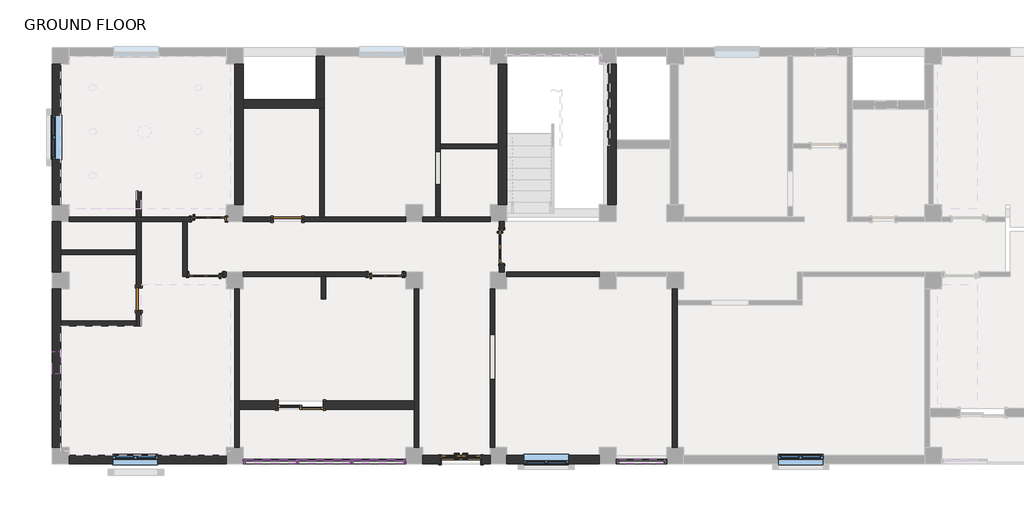
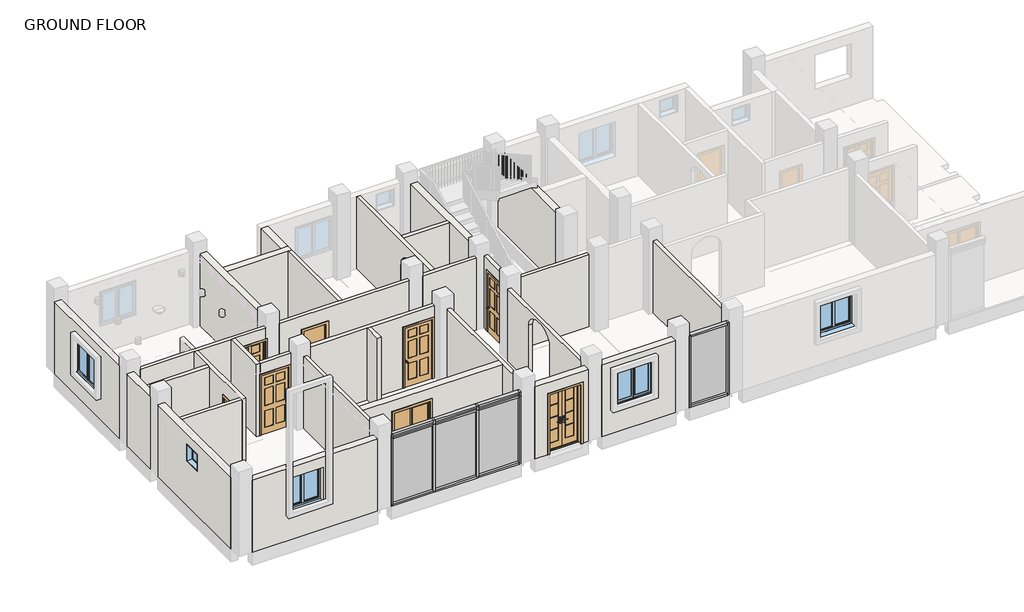
# One storey, part 1 of 5: 31 walls, 21 members, 8 doors, 7 plates, 5 windows.
"""IFC4 building model written with IfcOpenShell, lengths in millimetres."""

from ifc_helpers import new_model, si_unit, point, frame, origin, place, context, project, spatial, polyline, ellipse_curve, trimmed, outline, extrude, faceted_brep, transform, mapped, element, save
from ifc_brep_helpers import plane_surface, extruded_surface, advanced_brep
from components import door_double_sliding_4436dcad, door_exterior_double_full_glass_wood_clad_a9b2ee3b, door_c610b25b, door_03e3dfb5, single_flush_2_x_7_bath_room_door_025d1c86, door_e00f436c, member_f0fea5a5, member_ee409385, member_2b4cd6f1, member_0dc43c0c, member_71eb4692, member_9f3fc137, member_faf5b19b, member_68d3d74d, member_f51719be, member_c9ff5349, system_panel_glazed_7ffa2d15, system_panel_glazed_7e177a0b, system_panel_glazed_c89335d8, system_panel_glazed_a1658219, system_panel_glazed_dde0d99a, window_80340324, w2_0001_4_x_4_window_9dec5fc7

model = new_model("IFC4")

# Units and contexts
model_context = context("Model", 3, world=origin())
ifc_project = project(units=[si_unit("LENGTHUNIT", "METRE", prefix="MILLI")], contexts=[model_context])

# Site, building, storey
site = spatial("IfcSite", under=ifc_project)
building = spatial("IfcBuilding", under=site)
storey = spatial("IfcBuildingStorey", under=building, Name="GROUND FLOOR", Elevation=304.8)

# Doors
placement = place(None, origin())
door_double_sliding_shape = door_double_sliding_4436dcad(model_context)
element("IfcDoor", 1, ObjectType="Door-Double-Sliding", at=placement, inside=storey, context=model_context, shape_type="MappedRepresentation", body=[
    mapped(door_double_sliding_shape, transform((-8630.2456086, -9389.2679047, 304.8), x_axis=(-1.0, 0.0, 0.0), y_axis=(0.0, -1.0, 0.0), z_axis=(0.0, 0.0, 1.0))),
])
door_exterior_double_full_glass_wood_clad_shape = door_exterior_double_full_glass_wood_clad_a9b2ee3b(model_context)
element("IfcDoor", 2, ObjectType="Door-Exterior-Double-Full Glass-Wood_Clad", at=placement, inside=storey, context=model_context, shape_type="MappedRepresentation", body=[
    mapped(door_exterior_double_full_glass_wood_clad_shape, transform((-4274.1456086, -10998.9929047, 304.8), x_axis=(1.0, 0.0, 0.0), y_axis=(0.0, 1.0, 0.0), z_axis=(0.0, 0.0, 1.0))),
])
door_shape = door_c610b25b(model_context)
element("IfcDoor", 3, ObjectType="Door-Interior-Single-6_Panel-Wood : 36\" x 84\"", at=placement, inside=storey, context=model_context, shape_type="MappedRepresentation", body=[
    mapped(door_shape, transform((-6331.5456086, -5967.8544704, 304.8), x_axis=(1.0, 0.0, 0.0), y_axis=(0.0, 1.0, 0.0), z_axis=(0.0, 0.0, 1.0))),
])
element("IfcDoor", 4, ObjectType="Door-Interior-Single-6_Panel-Wood : 36\" x 84\"", at=placement, inside=storey, context=model_context, shape_type="MappedRepresentation", body=[
    mapped(door_shape, transform((-3172.4206086, -5215.3794704, 304.8), x_axis=(0.0, -1.0, 0.0), y_axis=(1.0, 0.0, 0.0), z_axis=(0.0, 0.0, 1.0))),
])
door_2_shape = door_03e3dfb5(model_context)
element("IfcDoor", 5, ObjectType="Door-Interior-Single-6_Panel-Wood : 36\" x 84\"", at=placement, inside=storey, context=model_context, shape_type="MappedRepresentation", body=[
    mapped(door_2_shape, transform((-11207.742897, -5967.8544704, 304.8), x_axis=(-1.0, 0.0, 0.0), y_axis=(0.0, -1.0, 0.0), z_axis=(0.0, 0.0, 1.0))),
])
element("IfcDoor", 6, ObjectType="Door-Interior-Single-6_Panel-Wood : 36\" x 84\"", at=placement, inside=storey, context=model_context, shape_type="MappedRepresentation", body=[
    mapped(door_2_shape, transform((-11132.1456086, -4462.9044704, 304.8), x_axis=(1.0, 0.0, 0.0), y_axis=(0.0, 1.0, 0.0), z_axis=(0.0, 0.0, 1.0))),
])
single_flush_2_x_7_bath_room_door_shape = single_flush_2_x_7_bath_room_door_025d1c86(model_context)
element("IfcDoor", 7, ObjectType="Single-Flush : 2' X 7' BATH ROOM DOOR", at=placement, inside=storey, context=model_context, shape_type="MappedRepresentation", body=[
    mapped(single_flush_2_x_7_bath_room_door_shape, transform((-13023.2401855, -6639.2659448, 304.8), x_axis=(0.0, 1.0, 0.0), y_axis=(-1.0, 0.0, 0.0), z_axis=(0.0, 0.0, 1.0))),
])
door_3_shape = door_e00f436c(model_context)
element("IfcDoor", 8, ObjectType="Single-Flush : bathroom 2'6\" door", at=placement, inside=storey, context=model_context, shape_type="MappedRepresentation", body=[
    mapped(door_3_shape, transform((-8985.8456086, -4466.0794704, 304.8), x_axis=(-1.0, 0.0, 0.0), y_axis=(0.0, -1.0, 0.0), z_axis=(0.0, 0.0, 1.0))),
])

# Members
member_shape = member_f0fea5a5(model_context)
element("IfcMember", 9, ObjectType="Rectangular Mullion : 2.5\" x 5\" rectangular", at=placement, inside=storey, context=model_context, shape_type="MappedRepresentation", body=[
    mapped(member_shape, transform((-8719.1456085, -11052.9679047, 304.8), x_axis=(1.0, 0.0, 0.0), y_axis=(0.0, -1.0, 0.0), z_axis=(0.0, 0.0, -1.0))),
])
element("IfcMember", 10, ObjectType="Rectangular Mullion : 2.5\" x 5\" rectangular", at=placement, inside=storey, context=model_context, shape_type="MappedRepresentation", body=[
    mapped(member_shape, transform((-7245.9456087, -11052.9679047, 304.8), x_axis=(1.0, 0.0, 0.0), y_axis=(0.0, -1.0, 0.0), z_axis=(0.0, 0.0, -1.0))),
])
member_2_shape = member_ee409385(model_context)
element("IfcMember", 11, ObjectType="Rectangular Mullion : 2.5\" x 5\" rectangular", at=placement, inside=storey, context=model_context, shape_type="MappedRepresentation", body=[
    mapped(member_2_shape, transform((-5772.7456086, -11052.9679047, 304.8), x_axis=(1.0, 0.0, 0.0), y_axis=(0.0, -1.0, 0.0), z_axis=(0.0, 0.0, -1.0))),
])
element("IfcMember", 12, ObjectType="Rectangular Mullion : 2.5\" x 5\" rectangular", at=placement, inside=storey, context=model_context, shape_type="MappedRepresentation", body=[
    mapped(member_2_shape, transform((-10192.3456086, -11052.9679047, 2743.2), x_axis=(-1.0, 0.0, 0.0), y_axis=(0.0, -1.0, 0.0), z_axis=(0.0, 0.0, 1.0))),
])
member_3_shape = member_2b4cd6f1(model_context)
element("IfcMember", 13, ObjectType="Rectangular Mullion : 2.5\" x 5\" rectangular", at=placement, inside=storey, context=model_context, shape_type="MappedRepresentation", body=[
    mapped(member_3_shape, transform((-5836.2456086, -11052.9679047, 2892.0191055), x_axis=(0.0, 0.0, 1.0), y_axis=(0.0, -1.0, 0.0), z_axis=(1.0, 0.0, 0.0))),
])
element("IfcMember", 14, ObjectType="Rectangular Mullion : 2.5\" x 5\" rectangular", at=placement, inside=storey, context=model_context, shape_type="MappedRepresentation", body=[
    mapped(member_3_shape, transform((-8750.8956085, -11052.9679047, 2892.0191055), x_axis=(0.0, 0.0, 1.0), y_axis=(0.0, -1.0, 0.0), z_axis=(1.0, 0.0, 0.0))),
])
element("IfcMember", 15, ObjectType="Rectangular Mullion : 2.5\" x 5\" rectangular", at=placement, inside=storey, context=model_context, shape_type="MappedRepresentation", body=[
    mapped(member_3_shape, transform((-10128.8456086, -11052.9679047, 304.8), x_axis=(0.0, 0.0, -1.0), y_axis=(0.0, -1.0, 0.0), z_axis=(-1.0, 0.0, 0.0))),
])
element("IfcMember", 16, ObjectType="Rectangular Mullion : 2.5\" x 5\" rectangular", at=placement, inside=storey, context=model_context, shape_type="MappedRepresentation", body=[
    mapped(member_3_shape, transform((-7214.1956087, -11052.9679047, 304.8), x_axis=(0.0, 0.0, -1.0), y_axis=(0.0, -1.0, 0.0), z_axis=(-1.0, 0.0, 0.0))),
])
member_4_shape = member_0dc43c0c(model_context)
element("IfcMember", 17, ObjectType="Rectangular Mullion : 2.5\" x 5\" rectangular", at=placement, inside=storey, context=model_context, shape_type="MappedRepresentation", body=[
    mapped(member_4_shape, transform((-7277.6956087, -11052.9679047, 2892.0191055), x_axis=(0.0, 0.0, 1.0), y_axis=(0.0, -1.0, 0.0), z_axis=(1.0, 0.0, 0.0))),
])
element("IfcMember", 18, ObjectType="Rectangular Mullion : 2.5\" x 5\" rectangular", at=placement, inside=storey, context=model_context, shape_type="MappedRepresentation", body=[
    mapped(member_4_shape, transform((-8687.3956085, -11052.9679047, 304.8), x_axis=(0.0, 0.0, -1.0), y_axis=(0.0, -1.0, 0.0), z_axis=(-1.0, 0.0, 0.0))),
])
member_5_shape = member_71eb4692(model_context)
element("IfcMember", 19, ObjectType="Rectangular Mullion : 2.5\" x 5\" rectangular", at=placement, inside=storey, context=model_context, shape_type="MappedRepresentation", body=[
    mapped(member_5_shape, transform((1246.8916602, -11052.9679047, 2895.6), x_axis=(0.0, 0.0, 1.0), y_axis=(0.0, -1.0, 0.0), z_axis=(1.0, 0.0, 0.0))),
])
element("IfcMember", 20, ObjectType="Rectangular Mullion : 2.5\" x 5\" rectangular", at=placement, inside=storey, context=model_context, shape_type="MappedRepresentation", body=[
    mapped(member_5_shape, transform((2.2916602, -11052.9679047, 304.8), x_axis=(0.0, 0.0, -1.0), y_axis=(0.0, -1.0, 0.0), z_axis=(-1.0, 0.0, 0.0))),
])
member_6_shape = member_9f3fc137(model_context)
element("IfcMember", 21, ObjectType="Rectangular Mullion : 2.5\" x 5\" rectangular", at=placement, inside=storey, context=model_context, shape_type="MappedRepresentation", body=[
    mapped(member_6_shape, transform((1310.3916602, -11052.9679047, 304.8), x_axis=(1.0, 0.0, 0.0), y_axis=(0.0, -1.0, 0.0), z_axis=(0.0, 0.0, -1.0))),
])
element("IfcMember", 22, ObjectType="Rectangular Mullion : 2.5\" x 5\" rectangular", at=placement, inside=storey, context=model_context, shape_type="MappedRepresentation", body=[
    mapped(member_6_shape, transform((-61.2083398, -11052.9679047, 2895.6), x_axis=(-1.0, 0.0, 0.0), y_axis=(0.0, -1.0, 0.0), z_axis=(0.0, 0.0, 1.0))),
])
member_7_shape = member_faf5b19b(model_context)
element("IfcMember", 23, ObjectType="Rectangular Mullion : 2.5\" x 5\" rectangular", at=placement, inside=storey, context=model_context, shape_type="MappedRepresentation", body=[
    mapped(member_7_shape, transform((-8750.8956085, -11052.9679047, 2743.2), x_axis=(0.0, 0.0, 1.0), y_axis=(0.0, -1.0, 0.0), z_axis=(1.0, 0.0, 0.0))),
])
element("IfcMember", 24, ObjectType="Rectangular Mullion : 2.5\" x 5\" rectangular", at=placement, inside=storey, context=model_context, shape_type="MappedRepresentation", body=[
    mapped(member_7_shape, transform((-5836.2456086, -11052.9679047, 2743.2), x_axis=(0.0, 0.0, 1.0), y_axis=(0.0, -1.0, 0.0), z_axis=(1.0, 0.0, 0.0))),
])
member_8_shape = member_68d3d74d(model_context)
element("IfcMember", 25, ObjectType="Rectangular Mullion : 2.5\" x 5\" rectangular", at=placement, inside=storey, context=model_context, shape_type="MappedRepresentation", body=[
    mapped(member_8_shape, transform((-7277.6956087, -11052.9679047, 2743.2), x_axis=(0.0, 0.0, 1.0), y_axis=(0.0, -1.0, 0.0), z_axis=(1.0, 0.0, 0.0))),
])
member_9_shape = member_f51719be(model_context)
element("IfcMember", 26, ObjectType="Rectangular Mullion : 2.5\" x 5\" rectangular", at=placement, inside=storey, context=model_context, shape_type="MappedRepresentation", body=[
    mapped(member_9_shape, transform((-8719.1456085, -11052.9679047, 2743.2), x_axis=(1.0, 0.0, 0.0), y_axis=(0.0, -1.0, 0.0), z_axis=(0.0, 0.0, -1.0))),
])
element("IfcMember", 27, ObjectType="Rectangular Mullion : 2.5\" x 5\" rectangular", at=placement, inside=storey, context=model_context, shape_type="MappedRepresentation", body=[
    mapped(member_9_shape, transform((-7245.9456087, -11052.9679047, 2743.2), x_axis=(1.0, 0.0, 0.0), y_axis=(0.0, -1.0, 0.0), z_axis=(0.0, 0.0, -1.0))),
])
member_10_shape = member_c9ff5349(model_context)
element("IfcMember", 28, ObjectType="Rectangular Mullion : 2.5\" x 5\" rectangular", at=placement, inside=storey, context=model_context, shape_type="MappedRepresentation", body=[
    mapped(member_10_shape, transform((-10192.3456086, -11052.9679047, 2892.0191055), x_axis=(-1.0, 0.0, 0.0), y_axis=(0.0, -1.0, 0.0), z_axis=(0.0, 0.0, 1.0))),
])
element("IfcMember", 29, ObjectType="Rectangular Mullion : 2.5\" x 5\" rectangular", at=placement, inside=storey, context=model_context, shape_type="MappedRepresentation", body=[
    mapped(member_10_shape, transform((-5772.7456086, -11052.9679047, 2743.2), x_axis=(1.0, 0.0, 0.0), y_axis=(0.0, -1.0, 0.0), z_axis=(0.0, 0.0, -1.0))),
])

# Plates
system_panel_glazed_shape = system_panel_glazed_7ffa2d15(model_context)
element("IfcPlate", 30, ObjectType="System Panel : Glazed", at=placement, inside=storey, context=model_context, shape_type="MappedRepresentation", body=[
    mapped(system_panel_glazed_shape, transform((624.5916602, -11052.9679047, 368.3), x_axis=(1.0, 0.0, 0.0), y_axis=(0.0, 1.0, 0.0), z_axis=(0.0, 0.0, 1.0))),
])
system_panel_glazed_2_shape = system_panel_glazed_7e177a0b(model_context)
element("IfcPlate", 31, ObjectType="System Panel : Glazed", at=placement, inside=storey, context=model_context, shape_type="MappedRepresentation", body=[
    mapped(system_panel_glazed_2_shape, transform((-9439.8706086, -11052.9679047, 368.3), x_axis=(1.0, 0.0, 0.0), y_axis=(0.0, 1.0, 0.0), z_axis=(0.0, 0.0, 1.0))),
])
element("IfcPlate", 32, ObjectType="System Panel : Glazed", at=placement, inside=storey, context=model_context, shape_type="MappedRepresentation", body=[
    mapped(system_panel_glazed_2_shape, transform((-6525.2206087, -11052.9679047, 368.3), x_axis=(1.0, 0.0, 0.0), y_axis=(0.0, 1.0, 0.0), z_axis=(0.0, 0.0, 1.0))),
])
system_panel_glazed_3_shape = system_panel_glazed_c89335d8(model_context)
element("IfcPlate", 33, ObjectType="System Panel : Glazed", at=placement, inside=storey, context=model_context, shape_type="MappedRepresentation", body=[
    mapped(system_panel_glazed_3_shape, transform((-7982.5456086, -11052.9679047, 368.3), x_axis=(1.0, 0.0, 0.0), y_axis=(0.0, 1.0, 0.0), z_axis=(0.0, 0.0, 1.0))),
])
system_panel_glazed_4_shape = system_panel_glazed_a1658219(model_context)
element("IfcPlate", 34, ObjectType="System Panel : Glazed", at=placement, inside=storey, context=model_context, shape_type="MappedRepresentation", body=[
    mapped(system_panel_glazed_4_shape, transform((-9439.8706086, -11052.9679047, 2774.95), x_axis=(1.0, 0.0, 0.0), y_axis=(0.0, 1.0, 0.0), z_axis=(0.0, 0.0, 1.0))),
])
element("IfcPlate", 35, ObjectType="System Panel : Glazed", at=placement, inside=storey, context=model_context, shape_type="MappedRepresentation", body=[
    mapped(system_panel_glazed_4_shape, transform((-6525.2206087, -11052.9679047, 2774.95), x_axis=(1.0, 0.0, 0.0), y_axis=(0.0, 1.0, 0.0), z_axis=(0.0, 0.0, 1.0))),
])
system_panel_glazed_5_shape = system_panel_glazed_dde0d99a(model_context)
element("IfcPlate", 36, ObjectType="System Panel : Glazed", at=placement, inside=storey, context=model_context, shape_type="MappedRepresentation", body=[
    mapped(system_panel_glazed_5_shape, transform((-7982.5456086, -11052.9679047, 2774.95), x_axis=(1.0, 0.0, 0.0), y_axis=(0.0, 1.0, 0.0), z_axis=(0.0, 0.0, 1.0))),
])

# Walls
element("IfcWall", 37, ObjectType="EXTERIOR WALL 9\"", at=placement, inside=storey, context=model_context, shape_type="SweptSolid", body=[
    extrude(outline(polyline([(304.8, -14916.7456086), (304.8, -10649.5456086), (2895.6, -10649.5456086), (2895.6, -14916.7456086), (304.8, -14916.7456086)]), holes=[polyline([(1304.8, -12503.7456086), (1304.8, -13722.9456086), (2524.0, -13722.9456086), (2524.0, -12503.7456086), (1304.8, -12503.7456086)])]), frame((0.0, -11116.4679047, 0.0), z_axis=(0.0, 1.0, 0.0), x_axis=(0.0, 0.0, 1.0)), (0.0, 0.0, 1.0), 228.6),
])
element("IfcWall", 38, ObjectType="EXTERIOR WALL 9\"", at=placement, inside=storey, context=model_context, shape_type="SweptSolid", body=[
    extrude(outline(polyline([(304.8, -3486.7456086), (2895.6, -3486.7456086), (2895.6, -5315.5456086), (304.8, -5315.5456086), (304.8, -4832.9456086), (2463.8, -4832.9456086), (2463.8, -3715.3456086), (304.8, -3715.3456086), (304.8, -3486.7456086)])), frame((0.0, -11116.4679047, 0.0), z_axis=(0.0, 1.0, 0.0), x_axis=(0.0, 0.0, 1.0)), (0.0, 0.0, 1.0), 228.6),
])
element("IfcWall", 39, ObjectType="EXTERIOR WALL 9\"", at=placement, inside=storey, context=model_context, shape_type="SweptSolid", body=[
    extrude(outline(polyline([(304.8, -3029.5456086), (304.8, -518.4083398), (2895.6, -518.4083398), (2895.6, -3029.5456086), (304.8, -3029.5456086)]), holes=[polyline([(1304.8, -2572.3456086), (2524.0, -2572.3456086), (2524.0, -1353.1456086), (1304.8, -1353.1456086), (1304.8, -2572.3456086)])]), frame((0.0, -11116.4679047, 0.0), z_axis=(0.0, 1.0, 0.0), x_axis=(0.0, 0.0, 1.0)), (0.0, 0.0, 1.0), 228.6),
])
element("IfcWall", 40, ObjectType="EXTERIOR WALL 9\"", at=placement, inside=storey, context=model_context, shape_type="Brep", body=[
    faceted_brep([(-15145.3456086, -10659.2679047, 304.8), (-15145.3456086, -7363.1659448, 304.8), (-15145.3456086, -7236.1659448, 304.8), (-15145.3456086, -6358.3794704, 304.8), (-15145.3456086, -6358.3794704, 2895.6), (-15145.3456086, -7236.1659448, 2895.6), (-15145.3456086, -7363.1659448, 2895.6), (-15145.3456086, -10659.2679047, 2895.6), (-15145.3456086, -8671.2659448, 2511.8263913), (-15145.3456086, -8061.6659448, 2511.8263913), (-15145.3456086, -8061.6659448, 1902.2263913), (-15145.3456086, -8671.2659448, 1902.2263913), (-15373.9456086, -10659.2679047, 304.8), (-15373.9456086, -10659.2679047, 2895.6), (-15373.9456086, -6358.3794704, 2895.6), (-15373.9456086, -6358.3794704, 304.8), (-15373.9456086, -8671.2659448, 2511.8263913), (-15373.9456086, -8671.2659448, 1902.2263913), (-15373.9456086, -8061.6659448, 1902.2263913), (-15373.9456086, -8061.6659448, 2511.8263913)], [[[0, 1, 2, 3, 4, 5, 6, 7], [8, 9, 10, 11]], [[12, 13, 14, 15], [16, 17, 18, 19]], [[3, 2, 1, 0, 12, 15]], [[4, 3, 15, 14]], [[7, 6, 5, 4, 14, 13]], [[0, 7, 13, 12]], [[17, 16, 8, 11]], [[18, 17, 11, 10]], [[19, 18, 10, 9]], [[16, 19, 9, 8]]]),
])
element("IfcWall", 41, ObjectType="EXTERIOR WALL 9\"", at=placement, inside=storey, context=model_context, shape_type="Brep", body=[
    faceted_brep([(-15145.3456086, -5901.1794704, 304.8), (-15145.3456086, -5431.2794704, 304.8), (-15145.3456086, -5304.2794704, 304.8), (-15145.3456086, -4529.5794704, 304.8), (-15145.3456086, -4529.5794704, 2895.6), (-15145.3456086, -5304.2794704, 2895.6), (-15145.3456086, -5431.2794704, 2895.6), (-15145.3456086, -5901.1794704, 2895.6), (-15373.9456086, -5901.1794704, 304.8), (-15373.9456086, -5901.1794704, 2895.6), (-15373.9456086, -4529.5794704, 2895.6), (-15373.9456086, -4529.5794704, 304.8)], [[[0, 1, 2, 3, 4, 5, 6, 7]], [[8, 9, 10, 11]], [[3, 2, 1, 0, 8, 11]], [[4, 3, 11, 10]], [[7, 6, 5, 4, 10, 9]], [[0, 7, 9, 8]]]),
])
element("IfcWall", 42, ObjectType="EXTERIOR WALL 9\"", at=placement, inside=storey, context=model_context, shape_type="SweptSolid", body=[
    extrude(outline(polyline([(-4072.3794704, 304.8), (-4072.3794704, 2895.6), (-262.3794704, 2895.6), (-262.3794704, 304.8), (-4072.3794704, 304.8)]), holes=[polyline([(-1633.9794704, 1219.2), (-1633.9794704, 2438.4), (-2853.1794704, 2438.4), (-2853.1794704, 1219.2), (-1633.9794704, 1219.2)])]), frame((-15373.9456086, 0.0, 0.0), z_axis=(1.0, 0.0, 0.0), x_axis=(0.0, 1.0, 0.0)), (0.0, 0.0, 1.0), 228.6),
])
element("IfcWall", 43, ObjectType="EXTERIOR WALL 9\"", at=placement, inside=storey, context=model_context, shape_type="Brep", body=[
    faceted_brep([(-10420.9456086, -262.3794704, 304.8), (-10420.9456086, -4072.3794704, 304.8), (-10420.9456086, -4072.3794704, 2895.6), (-10420.9456086, -262.3794704, 2895.6), (-10192.3456086, -262.3794704, 304.8), (-10192.3456086, -262.3794704, 2895.6), (-10192.3456086, -1214.8794704, 2895.6), (-10192.3456086, -1443.4794704, 2895.6), (-10192.3456086, -4072.3794704, 2895.6), (-10192.3456086, -4072.3794704, 304.8), (-10192.3456086, -1443.4794704, 304.8), (-10192.3456086, -1214.8794704, 304.8)], [[[0, 1, 2, 3]], [[4, 5, 6, 7, 8, 9, 10, 11]], [[1, 0, 4, 11, 10, 9]], [[2, 1, 9, 8]], [[3, 2, 8, 7, 6, 5]], [[0, 3, 5, 4]]]),
])
element("IfcWall", 44, ObjectType="EXTERIOR WALL 9\"", at=placement, inside=storey, context=model_context, shape_type="SweptSolid", body=[
    extrude(outline(polyline([(304.8, -10293.9456086), (304.8, -9239.8456086), (2438.4, -9239.8456086), (2438.4, -8020.6456086), (304.8, -8020.6456086), (304.8, -5544.1456086), (2895.6, -5544.1456086), (2895.6, -10293.9456086), (304.8, -10293.9456086)])), frame((0.0, -9630.5679047, 0.0), z_axis=(0.0, 1.0, 0.0), x_axis=(0.0, 0.0, 1.0)), (0.0, 0.0, 1.0), 228.6),
])
element("IfcWall", 45, ObjectType="EXTERIOR WALL 9\"", at=placement, inside=storey, context=model_context, shape_type="Brep", body=[
    faceted_brep([(-10192.3456086, -1443.4794704, 304.8), (-8109.5456086, -1443.4794704, 304.8), (-7982.5456086, -1443.4794704, 304.8), (-7982.5456086, -1443.4794704, 2895.6), (-8109.5456086, -1443.4794704, 2895.6), (-10192.3456086, -1443.4794704, 2895.6), (-10192.3456086, -1214.8794704, 304.8), (-10192.3456086, -1214.8794704, 2895.6), (-8211.1456086, -1214.8794704, 2895.6), (-7982.5456086, -1214.8794704, 2895.6), (-7982.5456086, -1214.8794704, 304.8), (-8211.1456086, -1214.8794704, 304.8)], [[[0, 1, 2, 3, 4, 5]], [[6, 7, 8, 9, 10, 11]], [[2, 1, 0, 6, 11, 10]], [[5, 4, 3, 9, 8, 7]], [[0, 5, 7, 6]], [[3, 2, 10, 9]]]),
])
element("IfcWall", 46, ObjectType="EXTERIOR WALL 9\"", at=placement, inside=storey, context=model_context, shape_type="SweptSolid", body=[
    extrude(outline(polyline([(-7982.5456086, -33.7794704), (-7982.5456086, -1214.8794704), (-8211.1456086, -1214.8794704), (-8211.1456086, -33.7794704), (-7982.5456086, -33.7794704)])), frame((0.0, 0.0, 304.8), z_axis=(0.0, 0.0, 1.0), x_axis=(1.0, 0.0, 0.0)), (0.0, 0.0, 1.0), 2590.8),
])
element("IfcWall", 47, ObjectType="EXTERIOR WALL 9\"", at=placement, inside=storey, context=model_context, shape_type="Brep", body=[
    faceted_brep([(-3258.1456086, -262.3794704, 304.8), (-3258.1456086, -2421.3794704, 304.8), (-3258.1456086, -2548.3794704, 304.8), (-3258.1456086, -4072.3794704, 304.8), (-3258.1456086, -4072.3794704, 2895.6), (-3258.1456086, -2548.3794704, 2895.6), (-3258.1456086, -2421.3794704, 2895.6), (-3258.1456086, -262.3794704, 2895.6), (-3029.5456086, -262.3794704, 304.8), (-3029.5456086, -262.3794704, 2895.6), (-3029.5456086, -4072.3794704, 2895.6), (-3029.5456086, -4072.3794704, 304.8)], [[[0, 1, 2, 3, 4, 5, 6, 7]], [[8, 9, 10, 11]], [[3, 2, 1, 0, 8, 11]], [[4, 3, 11, 10]], [[7, 6, 5, 4, 10, 9]], [[0, 7, 9, 8]]]),
])
element("IfcWall", 48, ObjectType="EXTERIOR WALL 9\"", at=placement, inside=storey, context=model_context, shape_type="Brep", body=[
    faceted_brep([(-289.8083398, -262.3794704, 304.8), (-289.8083398, -4072.3794704, 304.8), (-289.8083398, -4072.3794704, 2895.6), (-289.8083398, -262.3794704, 2895.6), (-61.2083398, -262.3794704, 304.8), (-61.2083398, -262.3794704, 2895.6), (-61.2083398, -2319.7794704, 2895.6), (-61.2083398, -2548.3794704, 2895.6), (-61.2083398, -4072.3794704, 2895.6), (-61.2083398, -4072.3794704, 304.8), (-61.2083398, -2548.3794704, 304.8), (-61.2083398, -2319.7794704, 304.8)], [[[0, 1, 2, 3]], [[4, 5, 6, 7, 8, 9, 10, 11]], [[1, 0, 4, 11, 10, 9]], [[2, 1, 9, 8]], [[3, 2, 8, 7, 6, 5]], [[0, 3, 5, 4]]]),
])
element("IfcWall", 49, ObjectType="INTERIOR WALL 5\"", at=placement, inside=storey, context=model_context, shape_type="Brep", body=[
    faceted_brep([(-10649.5456086, -4529.5794704, 2895.6), (-11702.4401855, -4529.5794704, 2895.6), (-11829.4401855, -4529.5794704, 2895.6), (-12959.7401855, -4529.5794704, 2895.6), (-13086.7401855, -4529.5794704, 2895.6), (-14916.7456086, -4529.5794704, 2895.6), (-14916.7456086, -4529.5794704, 304.8), (-13086.7401855, -4529.5794704, 304.8), (-12959.7401855, -4529.5794704, 304.8), (-11829.4401855, -4529.5794704, 304.8), (-11702.4401855, -4529.5794704, 304.8), (-11614.7456086, -4529.5794704, 304.8), (-11614.7456086, -4529.5794704, 2463.8), (-10649.5456086, -4529.5794704, 2463.8), (-14916.7456086, -4402.5794704, 2895.6), (-13086.7401855, -4402.5794704, 2895.6), (-12959.7401855, -4402.5794704, 2895.6), (-10649.5456086, -4402.5794704, 2895.6), (-10649.5456086, -4402.5794704, 2463.8), (-11614.7456086, -4402.5794704, 2463.8), (-11614.7456086, -4402.5794704, 304.8), (-12959.7401855, -4402.5794704, 304.8), (-13086.7401855, -4402.5794704, 304.8), (-14916.7456086, -4402.5794704, 304.8)], [[[0, 1, 2, 3, 4, 5, 6, 7, 8, 9, 10, 11, 12, 13]], [[14, 15, 16, 17, 18, 19, 20, 21, 22, 23]], [[6, 23, 22, 21, 20, 11, 10, 9, 8, 7]], [[17, 0, 13, 18]], [[5, 4, 3, 2, 1, 0, 17, 16, 15, 14]], [[6, 5, 14, 23]], [[12, 19, 18, 13]], [[19, 12, 11, 20]]]),
])
element("IfcWall", 50, ObjectType="INTERIOR WALL 5\"", at=placement, inside=storey, context=model_context, shape_type="Brep", body=[
    faceted_brep([(-13086.7401855, -3705.5659448, 2895.6), (-13086.7401855, -3705.5659448, 304.8), (-13086.7401855, -4402.5794704, 304.8), (-13086.7401855, -4402.5794704, 2895.6), (-12959.7401855, -3705.5659448, 304.8), (-12959.7401855, -3705.5659448, 2895.6), (-12959.7401855, -4402.5794704, 2895.6), (-12959.7401855, -4402.5794704, 304.8)], [[[0, 1, 2, 3]], [[4, 5, 6, 7]], [[1, 4, 7, 2]], [[5, 0, 3, 6]], [[1, 0, 5, 4]], [[3, 2, 7, 6]]]),
    faceted_brep([(-13086.7401855, -7363.1659448, 304.8), (-13086.7401855, -7363.1659448, 2895.6), (-13086.7401855, -7236.1659448, 2895.6), (-13086.7401855, -5431.2794704, 2895.6), (-13086.7401855, -5304.2794704, 2895.6), (-13086.7401855, -4529.5794704, 2895.6), (-13086.7401855, -4529.5794704, 304.8), (-13086.7401855, -5304.2794704, 304.8), (-13086.7401855, -5431.2794704, 304.8), (-13086.7401855, -6334.4659448, 304.8), (-13086.7401855, -6334.4659448, 2336.8), (-13086.7401855, -6944.0659448, 2336.8), (-13086.7401855, -6944.0659448, 304.8), (-13086.7401855, -7236.1659448, 304.8), (-12959.7401855, -7363.1659448, 2895.6), (-12959.7401855, -7363.1659448, 304.8), (-12959.7401855, -6944.0659448, 304.8), (-12959.7401855, -6944.0659448, 2336.8), (-12959.7401855, -6334.4659448, 2336.8), (-12959.7401855, -6334.4659448, 304.8), (-12959.7401855, -4529.5794704, 304.8), (-12959.7401855, -4529.5794704, 2895.6)], [[[0, 1, 2, 3, 4, 5, 6, 7, 8, 9, 10, 11, 12, 13]], [[14, 15, 16, 17, 18, 19, 20, 21]], [[15, 0, 13, 12, 16]], [[19, 9, 8, 7, 6, 20]], [[1, 14, 21, 5, 4, 3, 2]], [[6, 5, 21, 20]], [[1, 0, 15, 14]], [[10, 9, 19, 18]], [[11, 10, 18, 17]], [[12, 11, 17, 16]]]),
])
element("IfcWall", 51, ObjectType="INTERIOR WALL 5\"", at=placement, inside=storey, context=model_context, shape_type="SweptSolid", body=[
    extrude(outline(polyline([(-15145.3456086, -7236.1659448), (-13086.7401855, -7236.1659448), (-13086.7401855, -7363.1659448), (-15145.3456086, -7363.1659448), (-15145.3456086, -7236.1659448)])), frame((0.0, 0.0, 304.8), z_axis=(0.0, 0.0, 1.0), x_axis=(1.0, 0.0, 0.0)), (0.0, 0.0, 1.0), 2590.8),
])
element("IfcWall", 52, ObjectType="INTERIOR WALL 5\"", at=placement, inside=storey, context=model_context, shape_type="SweptSolid", body=[
    extrude(outline(polyline([(-13086.7401855, -5431.2794704), (-15145.3456086, -5431.2794704), (-15145.3456086, -5304.2794704), (-13086.7401855, -5304.2794704), (-13086.7401855, -5431.2794704)])), frame((0.0, 0.0, 304.8), z_axis=(0.0, 0.0, 1.0), x_axis=(1.0, 0.0, 0.0)), (0.0, 0.0, 1.0), 2590.8),
])
element("IfcWall", 53, ObjectType="INTERIOR WALL 5\"", at=placement, inside=storey, context=model_context, shape_type="Brep", body=[
    faceted_brep([(-10293.9456086, -10659.2679047, 304.8), (-10293.9456086, -9630.5679047, 304.8), (-10293.9456086, -9401.9679047, 304.8), (-10293.9456086, -6358.3794704, 304.8), (-10293.9456086, -6358.3794704, 2895.6), (-10293.9456086, -9401.9679047, 2895.6), (-10293.9456086, -9630.5679047, 2895.6), (-10293.9456086, -10659.2679047, 2895.6), (-10420.9456086, -10659.2679047, 304.8), (-10420.9456086, -10659.2679047, 2895.6), (-10420.9456086, -6358.3794704, 2895.6), (-10420.9456086, -6358.3794704, 304.8)], [[[0, 1, 2, 3, 4, 5, 6, 7]], [[8, 9, 10, 11]], [[3, 2, 1, 0, 8, 11]], [[4, 3, 11, 10]], [[7, 6, 5, 4, 10, 9]], [[0, 7, 9, 8]]]),
])
element("IfcWall", 54, ObjectType="INTERIOR WALL 5\"", at=placement, inside=storey, context=model_context, shape_type="Brep", body=[
    faceted_brep([(-10192.3456086, -5901.1794704, 304.8), (-10192.3456086, -5901.1794704, 2895.6), (-5772.7456086, -5901.1794704, 2895.6), (-5772.7456086, -5901.1794704, 304.8), (-5848.9456086, -5901.1794704, 304.8), (-5848.9456086, -5901.1794704, 2463.8), (-6814.1456086, -5901.1794704, 2463.8), (-6814.1456086, -5901.1794704, 304.8), (-10192.3456086, -6028.1794704, 2895.6), (-10192.3456086, -6028.1794704, 304.8), (-8071.4456086, -6028.1794704, 304.8), (-7944.4456086, -6028.1794704, 304.8), (-6814.1456086, -6028.1794704, 304.8), (-6814.1456086, -6028.1794704, 2463.8), (-5848.9456086, -6028.1794704, 2463.8), (-5848.9456086, -6028.1794704, 304.8), (-5772.7456086, -6028.1794704, 304.8), (-5772.7456086, -6028.1794704, 2895.6), (-7944.4456086, -6028.1794704, 2895.6), (-8071.4456086, -6028.1794704, 2895.6)], [[[0, 1, 2, 3, 4, 5, 6, 7]], [[8, 9, 10, 11, 12, 13, 14, 15, 16, 17, 18, 19]], [[9, 0, 7, 12, 11, 10]], [[3, 16, 15, 4]], [[1, 0, 9, 8]], [[2, 1, 8, 19, 18, 17]], [[3, 2, 17, 16]], [[14, 5, 4, 15]], [[5, 14, 13, 6]], [[6, 13, 12, 7]]]),
])
element("IfcWall", 55, ObjectType="INTERIOR WALL 5\"", at=placement, inside=storey, context=model_context, shape_type="SweptSolid", body=[
    extrude(outline(polyline([(-8071.4456086, -6637.7794704), (-8071.4456086, -6028.1794704), (-7944.4456086, -6028.1794704), (-7944.4456086, -6637.7794704), (-8071.4456086, -6637.7794704)])), frame((0.0, 0.0, 304.8), z_axis=(0.0, 0.0, 1.0), x_axis=(1.0, 0.0, 0.0)), (0.0, 0.0, 1.0), 2590.8),
])
element("IfcWall", 56, ObjectType="INTERIOR WALL 5\"", at=placement, inside=storey, context=model_context, shape_type="Brep", body=[
    faceted_brep([(-5417.1456086, -10659.2679047, 304.8), (-5417.1456086, -6358.3794704, 304.8), (-5417.1456086, -6358.3794704, 2895.6), (-5417.1456086, -10659.2679047, 2895.6), (-5544.1456086, -10659.2679047, 304.8), (-5544.1456086, -10659.2679047, 2895.6), (-5544.1456086, -9630.5679047, 2895.6), (-5544.1456086, -9401.9679047, 2895.6), (-5544.1456086, -6358.3794704, 2895.6), (-5544.1456086, -6358.3794704, 304.8), (-5544.1456086, -9401.9679047, 304.8), (-5544.1456086, -9630.5679047, 304.8)], [[[0, 1, 2, 3]], [[4, 5, 6, 7, 8, 9, 10, 11]], [[1, 0, 4, 11, 10, 9]], [[2, 1, 9, 8]], [[3, 2, 8, 7, 6, 5]], [[0, 3, 5, 4]]]),
])
element("IfcWall", 57, ObjectType="INTERIOR WALL 5\"", at=placement, inside=storey, context=model_context, shape_type="AdvancedBrep", body=[
    advanced_brep(
    [(-3486.7456086, -10659.2679047, 304.8), (-3486.7456086, -10659.2679047, 2895.6), (-3486.7456086, -6358.3794704, 2895.6), (-3486.7456086, -6358.3794704, 304.8), (-3486.7456086, -7604.4016919, 2349.6631591), (-3486.7456086, -8823.6016919, 2349.6631591), (-3486.7456086, -8823.6016919, 393.8631591), (-3486.7456086, -7604.4016919, 393.8631591), (-3359.7456086, -10659.2679047, 304.8), (-3359.7456086, -6358.3794704, 304.8), (-3359.7456086, -6358.3794704, 2895.6), (-3359.7456086, -10659.2679047, 2895.6), (-3359.7456086, -7604.4016919, 2349.6631591), (-3359.7456086, -7604.4016919, 393.8631591), (-3359.7456086, -8823.6016919, 393.8631591), (-3359.7456086, -8823.6016919, 2349.6631591)],
    [
        (0, 1),
        (1, 2),
        (2, 3),
        (3, 0),
        (4, 5, ellipse_curve(frame((-3486.7456086, -8214.0016919, 2349.6631591), z_axis=(1.0, 0.0, 0.0), x_axis=(0.0, -1.0, 0.0)), 609.6, 457.2)),
        (5, 6),
        (6, 7),
        (7, 4),
        (8, 9),
        (9, 10),
        (10, 11),
        (11, 8),
        (12, 13),
        (13, 14),
        (14, 15),
        (15, 12, ellipse_curve(frame((-3359.7456086, -8214.0016919, 2349.6631591), z_axis=(-1.0, 0.0, 0.0), x_axis=(0.0, -1.0, 0.0)), 609.6, 457.2)),
        (3, 9),
        (8, 0),
        (11, 1),
        (10, 2),
        (4, 12),
        (15, 5),
        (14, 6),
        (13, 7),
    ],
    [
        plane_surface(frame((-3486.7456086, -10659.2679047, 304.8), z_axis=(-1.0, 0.0, 0.0), x_axis=(0.0, 0.0, 1.0))),
        plane_surface(frame((-3359.7456086, -10659.2679047, 304.8), z_axis=(1.0, 0.0, 0.0), x_axis=(0.0, 0.0, -1.0))),
        plane_surface(frame((-3486.7456086, -6358.3794704, 304.8), z_axis=(0.0, 0.0, -1.0), x_axis=(1.0, 0.0, 0.0))),
        plane_surface(frame((-3486.7456086, -10659.2679047, 304.8), z_axis=(0.0, -1.0, 0.0), x_axis=(1.0, 0.0, 0.0))),
        plane_surface(frame((-3486.7456086, -10659.2679047, 2895.6), z_axis=(0.0, 0.0, 1.0), x_axis=(1.0, 0.0, 0.0))),
        plane_surface(frame((-3486.7456086, -6358.3794704, 2895.6), z_axis=(0.0, 1.0, 0.0), x_axis=(1.0, 0.0, 0.0))),
        extruded_surface(trimmed(ellipse_curve(frame((-3296.2456086, -8214.0016919, 2349.6631591), z_axis=(1.0, 0.0, 0.0), x_axis=(0.0, -1.0, 0.0)), 609.6, 457.2), [point((-3296.2456086, -7604.4016919, 2349.6631591))], [point((-3296.2456086, -8823.6016919, 2349.6631591))], True, "CARTESIAN"), (-127.0, 0.0, 0.0), 127.0),
        plane_surface(frame((-3486.7456086, -8823.6016919, 2349.6631591), z_axis=(0.0, 1.0, 0.0), x_axis=(1.0, 0.0, 0.0))),
        plane_surface(frame((-3486.7456086, -8823.6016919, 393.8631591), z_axis=(0.0, 0.0, 1.0), x_axis=(1.0, 0.0, 0.0))),
        plane_surface(frame((-3486.7456086, -7604.4016919, 393.8631591), z_axis=(0.0, -1.0, 0.0), x_axis=(1.0, 0.0, 0.0))),
    ],
    [
        (0, [[1, 2, 3, 4], [5, 6, 7, 8]]),
        (1, [[9, 10, 11, 12], [13, 14, 15, 16]]),
        (2, [[-4, 17, -9, 18]]),
        (3, [[-1, -18, -12, 19]]),
        (4, [[-2, -19, -11, 20]]),
        (5, [[-3, -20, -10, -17]]),
        (6, [[-5, 21, -16, 22]]),
        (7, [[-6, -22, -15, 23]]),
        (8, [[-7, -23, -14, 24]]),
        (9, [[-8, -24, -13, -21]]),
    ],
),
])
element("IfcWall", 58, ObjectType="INTERIOR WALL 5\"", at=placement, inside=storey, context=model_context, shape_type="Brep", body=[
    faceted_brep([(1589.7916602, -10659.2679047, 304.8), (1589.7916602, -6802.8794704, 304.8), (1589.7916602, -6675.8794704, 304.8), (1589.7916602, -6358.3794704, 304.8), (1589.7916602, -6358.3794704, 2895.6), (1589.7916602, -6675.8794704, 2895.6), (1589.7916602, -6802.8794704, 2895.6), (1589.7916602, -10659.2679047, 2895.6), (1462.7916602, -10659.2679047, 304.8), (1462.7916602, -10659.2679047, 2895.6), (1462.7916602, -6358.3794704, 2895.6), (1462.7916602, -6358.3794704, 304.8)], [[[0, 1, 2, 3, 4, 5, 6, 7]], [[8, 9, 10, 11]], [[3, 2, 1, 0, 8, 11]], [[4, 3, 11, 10]], [[7, 6, 5, 4, 10, 9]], [[0, 7, 9, 8]]]),
])
element("IfcWall", 59, ObjectType="INTERIOR WALL 5\"", at=placement, inside=storey, context=model_context, shape_type="Brep", body=[
    faceted_brep([(-10192.3456086, -4529.5794704, 304.8), (-9366.8456086, -4529.5794704, 304.8), (-9366.8456086, -4529.5794704, 2336.8), (-8604.8456086, -4529.5794704, 2336.8), (-8604.8456086, -4529.5794704, 304.8), (-5772.7456086, -4529.5794704, 304.8), (-5772.7456086, -4529.5794704, 2895.6), (-10192.3456086, -4529.5794704, 2895.6), (-9366.8456086, -4402.5794704, 2336.8), (-9366.8456086, -4402.5794704, 304.8), (-10192.3456086, -4402.5794704, 304.8), (-10192.3456086, -4402.5794704, 2895.6), (-8109.5456086, -4402.5794704, 2895.6), (-7982.5456086, -4402.5794704, 2895.6), (-5772.7456086, -4402.5794704, 2895.6), (-5772.7456086, -4402.5794704, 304.8), (-7982.5456086, -4402.5794704, 304.8), (-8109.5456086, -4402.5794704, 304.8), (-8604.8456086, -4402.5794704, 304.8), (-8604.8456086, -4402.5794704, 2336.8)], [[[0, 1, 2, 3, 4, 5, 6, 7]], [[8, 9, 10, 11, 12, 13, 14, 15, 16, 17, 18, 19]], [[10, 9, 1, 0]], [[18, 17, 16, 15, 5, 4]], [[6, 5, 15, 14]], [[7, 6, 14, 13, 12, 11]], [[0, 7, 11, 10]], [[2, 1, 9, 8]], [[3, 2, 8, 19]], [[4, 3, 19, 18]]]),
])
element("IfcWall", 60, ObjectType="INTERIOR WALL 5\"", at=placement, inside=storey, context=model_context, shape_type="Brep", body=[
    faceted_brep([(-5315.5456086, -4529.5794704, 304.8), (-3486.7456086, -4529.5794704, 304.8), (-3486.7456086, -4529.5794704, 2895.6), (-5315.5456086, -4529.5794704, 2895.6), (-5315.5456086, -4402.5794704, 304.8), (-5315.5456086, -4402.5794704, 2895.6), (-4959.9456086, -4402.5794704, 2895.6), (-4832.9456086, -4402.5794704, 2895.6), (-3486.7456086, -4402.5794704, 2895.6), (-3486.7456086, -4402.5794704, 304.8), (-4832.9456086, -4402.5794704, 304.8), (-4959.9456086, -4402.5794704, 304.8)], [[[0, 1, 2, 3]], [[4, 5, 6, 7, 8, 9, 10, 11]], [[1, 0, 4, 11, 10, 9]], [[2, 1, 9, 8]], [[3, 2, 8, 7, 6, 5]], [[0, 3, 5, 4]]]),
])
element("IfcWall", 61, ObjectType="INTERIOR WALL 5\"", at=placement, inside=storey, context=model_context, shape_type="SweptSolid", body=[
    extrude(outline(polyline([(-8109.5456086, -4402.5794704), (-8109.5456086, -1443.4794704), (-7982.5456086, -1443.4794704), (-7982.5456086, -4402.5794704), (-8109.5456086, -4402.5794704)])), frame((0.0, 0.0, 304.8), z_axis=(0.0, 0.0, 1.0), x_axis=(1.0, 0.0, 0.0)), (0.0, 0.0, 1.0), 2590.8),
])
element("IfcWall", 62, ObjectType="INTERIOR WALL 5\"", at=placement, inside=storey, context=model_context, shape_type="AdvancedBrep", body=[
    advanced_brep(
    [(-4959.9456086, -33.7794704, 304.8), (-4959.9456086, -4402.5794704, 304.8), (-4959.9456086, -4402.5794704, 2895.6), (-4959.9456086, -33.7794704, 2895.6), (-4959.9456086, -3525.9205586, 1993.0197979), (-4959.9456086, -3525.9205586, 367.4197979), (-4959.9456086, -2636.9205586, 367.4197979), (-4959.9456086, -2636.9205586, 1993.0197979), (-4832.9456086, -33.7794704, 304.8), (-4832.9456086, -33.7794704, 2895.6), (-4832.9456086, -2421.3794704, 2895.6), (-4832.9456086, -2548.3794704, 2895.6), (-4832.9456086, -4402.5794704, 2895.6), (-4832.9456086, -4402.5794704, 304.8), (-4832.9456086, -2548.3794704, 304.8), (-4832.9456086, -2421.3794704, 304.8), (-4832.9456086, -3525.9205586, 1993.0197979), (-4832.9456086, -2636.9205586, 1993.0197979), (-4832.9456086, -2636.9205586, 367.4197979), (-4832.9456086, -3525.9205586, 367.4197979)],
    [
        (0, 1),
        (1, 2),
        (2, 3),
        (3, 0),
        (4, 5),
        (5, 6),
        (6, 7),
        (7, 4, ellipse_curve(frame((-4959.9456086, -3081.4205586, 1993.0197979), z_axis=(1.0, 0.0, 0.0), x_axis=(0.0, 0.0, 1.0)), 482.6, 444.5)),
        (8, 9),
        (9, 10),
        (10, 11),
        (11, 12),
        (12, 13),
        (13, 14),
        (14, 15),
        (15, 8),
        (16, 17, ellipse_curve(frame((-4832.9456086, -3081.4205586, 1993.0197979), z_axis=(-1.0, 0.0, 0.0), x_axis=(0.0, 0.0, 1.0)), 482.6, 444.5)),
        (17, 18),
        (18, 19),
        (19, 16),
        (3, 9),
        (8, 0),
        (1, 13),
        (12, 2),
        (4, 16),
        (19, 5),
        (18, 6),
        (17, 7),
    ],
    [
        plane_surface(frame((-4959.9456086, -33.7794704, 304.8), z_axis=(-1.0, 0.0, 0.0), x_axis=(0.0, -1.0, 0.0))),
        plane_surface(frame((-4832.9456086, -33.7794704, 304.8), z_axis=(1.0, 0.0, 0.0), x_axis=(0.0, 1.0, 0.0))),
        plane_surface(frame((-5296.6260942, -33.7794704, 304.8), z_axis=(0.0, 1.0, 0.0), x_axis=(1.0, 0.0, 0.0))),
        plane_surface(frame((-5315.5456086, -4402.5794704, 304.8), z_axis=(0.0, -1.0, 0.0), x_axis=(-1.0, 0.0, 0.0))),
        plane_surface(frame((-4959.9456086, 80.5205296, 304.8), z_axis=(0.0, 0.0, -1.0), x_axis=(1.0, 0.0, 0.0))),
        plane_surface(frame((-4959.9456086, -4466.0794704, 2895.6), z_axis=(0.0, 0.0, 1.0), x_axis=(1.0, 0.0, 0.0))),
        plane_surface(frame((-4959.9456086, -3525.9205586, 1993.0197979), z_axis=(0.0, 1.0, 0.0), x_axis=(1.0, 0.0, 0.0))),
        plane_surface(frame((-4959.9456086, -3525.9205586, 367.4197979), z_axis=(0.0, 0.0, 1.0), x_axis=(1.0, 0.0, 0.0))),
        plane_surface(frame((-4959.9456086, -2636.9205586, 367.4197979), z_axis=(0.0, -1.0, 0.0), x_axis=(1.0, 0.0, 0.0))),
        extruded_surface(trimmed(ellipse_curve(frame((-4769.4456086, -3081.4205586, 1993.0197979), z_axis=(1.0, 0.0, 0.0), x_axis=(0.0, 1.0, 0.0)), 444.5, 482.6), [point((-4769.4456086, -2636.9205586, 1993.0197979))], [point((-4769.4456086, -3525.9205586, 1993.0197979))], True, "CARTESIAN"), (-127.0, 0.0, 0.0), 127.0),
    ],
    [
        (0, [[1, 2, 3, 4], [5, 6, 7, 8]]),
        (1, [[9, 10, 11, 12, 13, 14, 15, 16], [17, 18, 19, 20]]),
        (2, [[-4, 21, -9, 22]]),
        (3, [[-2, 23, -13, 24]]),
        (4, [[-1, -22, -16, -15, -14, -23]]),
        (5, [[-3, -24, -12, -11, -10, -21]]),
        (6, [[-5, 25, -20, 26]]),
        (7, [[-6, -26, -19, 27]]),
        (8, [[-7, -27, -18, 28]]),
        (9, [[-8, -28, -17, -25]]),
    ],
),
])
element("IfcWall", 63, ObjectType="INTERIOR WALL 5\"", at=placement, inside=storey, context=model_context, shape_type="SweptSolid", body=[
    extrude(outline(polyline([(-3258.1456086, -2548.3794704), (-4832.9456086, -2548.3794704), (-4832.9456086, -2421.3794704), (-3258.1456086, -2421.3794704), (-3258.1456086, -2548.3794704)])), frame((0.0, 0.0, 304.8), z_axis=(0.0, 0.0, 1.0), x_axis=(1.0, 0.0, 0.0)), (0.0, 0.0, 1.0), 2590.8),
])
element("IfcWall", 64, ObjectType="INTERIOR WALL 5\"", at=placement, inside=storey, context=model_context, shape_type="SweptSolid", body=[
    extrude(outline(polyline([(-3029.5456086, -5901.1794704), (-518.4083398, -5901.1794704), (-518.4083398, -6028.1794704), (-3029.5456086, -6028.1794704), (-3029.5456086, -5901.1794704)])), frame((0.0, 0.0, 304.8), z_axis=(0.0, 0.0, 1.0), x_axis=(1.0, 0.0, 0.0)), (0.0, 0.0, 1.0), 2590.8),
])
element("IfcWall", 65, ObjectType="INTERIOR WALL 5\"", at=placement, inside=storey, context=model_context, shape_type="SweptSolid", body=[
    extrude(outline(polyline([(-5901.1794704, 304.8), (-5901.1794704, 2895.6), (-4529.5794704, 2895.6), (-4529.5794704, 304.8), (-4732.7794704, 304.8), (-4732.7794704, 2463.8), (-5697.9794704, 2463.8), (-5697.9794704, 304.8), (-5901.1794704, 304.8)])), frame((-3232.7456086, 0.0, 0.0), z_axis=(1.0, 0.0, 0.0), x_axis=(0.0, 1.0, 0.0)), (0.0, 0.0, 1.0), 127.0),
])
element("IfcWall", 66, ObjectType="INTERIOR WALL 5\"", at=placement, inside=storey, context=model_context, shape_type="Brep", body=[
    faceted_brep([(-11829.4401855, -4529.5794704, 304.8), (-11829.4401855, -6028.1794704, 304.8), (-11829.4401855, -6028.1794704, 2895.6), (-11829.4401855, -4529.5794704, 2895.6), (-11702.4401855, -4529.5794704, 304.8), (-11702.4401855, -4529.5794704, 2895.6), (-11702.4401855, -5901.1794704, 2895.6), (-11702.4401855, -6028.1794704, 2895.6), (-11702.4401855, -6028.1794704, 304.8), (-11702.4401855, -5901.1794704, 304.8)], [[[0, 1, 2, 3]], [[4, 5, 6, 7, 8, 9]], [[1, 0, 4, 9, 8]], [[3, 2, 7, 6, 5]], [[0, 3, 5, 4]], [[2, 1, 8, 7]]]),
])
element("IfcWall", 67, ObjectType="INTERIOR WALL 5\"", at=placement, inside=storey, context=model_context, shape_type="SweptSolid", body=[
    extrude(outline(polyline([(2895.6, -10649.5456086), (2895.6, -11702.4401855), (304.8, -11702.4401855), (304.8, -11690.342897), (2463.8, -11690.342897), (2463.8, -10725.142897), (304.8, -10725.142897), (304.8, -10649.5456086), (2895.6, -10649.5456086)])), frame((0.0, -6028.1794704, 0.0), z_axis=(0.0, 1.0, 0.0), x_axis=(0.0, 0.0, 1.0)), (0.0, 0.0, 1.0), 127.0),
])

# Windows
window_shape = window_80340324(model_context)
element("IfcWindow", 68, ObjectType="Fixed : 24\" x 24\"", at=placement, inside=storey, context=model_context, shape_type="MappedRepresentation", body=[
    mapped(window_shape, transform((-15259.6456086, -8404.5659448, 987.8263913), x_axis=(0.0, -1.0, 0.0), y_axis=(1.0, 0.0, 0.0), z_axis=(0.0, 0.0, 1.0))),
])
w2_0001_4_x_4_window_shape = w2_0001_4_x_4_window_9dec5fc7(model_context)
element("IfcWindow", 69, ObjectType="w2.0001 : 4' X 4' WINDOW", at=placement, inside=storey, context=model_context, shape_type="MappedRepresentation", body=[
    mapped(w2_0001_4_x_4_window_shape, transform((-13113.3456086, -11002.1679047, 304.8), x_axis=(-1.0, 0.0, 0.0), y_axis=(0.0, -1.0, 0.0), z_axis=(0.0, 0.0, 1.0))),
])
element("IfcWindow", 70, ObjectType="w2.0001 : 4' X 4' WINDOW", at=placement, inside=storey, context=model_context, shape_type="MappedRepresentation", body=[
    mapped(w2_0001_4_x_4_window_shape, transform((4942.5916602, -11002.1679047, 304.8), x_axis=(-1.0, 0.0, 0.0), y_axis=(0.0, -1.0, 0.0), z_axis=(0.0, 0.0, 1.0))),
])
element("IfcWindow", 71, ObjectType="w2.0001 : 4' X 4' WINDOW", at=placement, inside=storey, context=model_context, shape_type="MappedRepresentation", body=[
    mapped(w2_0001_4_x_4_window_shape, transform((-1962.7456086, -11002.1679047, 304.8), x_axis=(1.0, 0.0, 0.0), y_axis=(0.0, 1.0, 0.0), z_axis=(0.0, 0.0, 1.0))),
])
element("IfcWindow", 72, ObjectType="w2.0001 : 4' X 4' WINDOW", at=placement, inside=storey, context=model_context, shape_type="MappedRepresentation", body=[
    mapped(w2_0001_4_x_4_window_shape, transform((-15259.6456086, -2243.5794704, 219.2), x_axis=(0.0, -1.0, 0.0), y_axis=(1.0, 0.0, 0.0), z_axis=(0.0, 0.0, 1.0))),
])

save(model, "model.ifc")

# Revit data of these elements
# Type "Door-Double-Sliding"
#   Type Mark = "14"
#   Construction Type Id = "opn-d45"
#   Assembly Code = "C1020"
#   Analytic Construction = "Wood frame, double glass door "
#   Thickness = 0' - 2"
#   Thermal Resistance (R) = 1.8150 (h·ft²·°F)/BTU
#   Heat Transfer Coefficient (U) = 0.5510 BTU/(h·ft²·°F)
#   Height = 7' - 0"
#   Rail Width = 0' - 2"
#   Stiles = 0' - 2"
#   Trim Projection Ext = 0' - 1"
#   Trim Projection Int = 0' - 1"
#   Trim Width = 0' - 3"
#   Width = 4' - 0"
#   Define Thermal Properties by = 1
#   Glazing = Glass
#   Panel Material = Wood - Birch - Solid Stained Light Low Gloss
#   Trim Material = Paint - Sienna
#   Visual Light Transmittance = 0
#   Solar Heat Gain Coefficient = 0
#   Function = (empty or 0)
#   Wall Closure = (empty or 0)
# Type "Door-Exterior-Double-Full Glass-Wood_Clad"
#   Type Mark = "9"
#   Assembly Code = "B2030100"
#   Analytic Construction = "French door, wood frame with double glass"
#   Top Rail = 0' - 4 11/16"
#   Threshold Offset [instance default] = 0' - 0 1/2"
#   Thickness = 0' - 1 3/8"
#   Thermal Resistance (R) = 1.9158 (h·ft²·°F)/BTU
#   Swing Angle [instance default] = 90.00°
#   Stiles = 0' - 4 3/4"
#   Rough Width = 3' - 8"
#   Rough Height = 7' - 1"
#   Panel Width = 1' - 9"
#   Door Offset [instance default] = 0' - 0"
#   Height = 7' - 0"
#   Width = 3' - 6"
#   Heat Transfer Coefficient (U) = 0.5220 BTU/(h·ft²·°F)
#   Bottom Rail = 0' - 9 1/8"
#   Exterior Trim [instance default] = yes
#   Threshold [instance default] = yes
#   Show Grill [instance default] = yes
#   Function = 1
#   Trim Material = Cherry
#   Threshold Material = Cherry
#   Panel Material = Cherry
#   Glazing = Glass
#   Frame Material = Cherry
#   Door Handle Material = Aluminum
#   Visual Light Transmittance = 0
#   Solar Heat Gain Coefficient = 0
#   Wall Closure = (empty or 0)
#   Construction Type = (empty or 0)
# Type "Door-Interior-Single-6_Panel-Wood : 36\" x 84\""
#   Type Mark = "10"
#   Assembly Code = "C1020300"
#   Analytic Construction = "Wooden"
#   Top Rail = 0' - 4 11/16"
#   Top Panel = 0' - 11"
#   Thickness = 0' - 1 3/8"
#   Thermal Resistance (R) = 2.5876 (h·ft²·°F)/BTU
#   Swing Angle [instance default] = 90.00°
#   Stiles = 0' - 4 3/4"
#   Rough Width = 3' - 2"
#   Rough Height = 7' - 1"
#   Mullion = 0' - 4 1/2"
#   Lock Rail = 0' - 7 1/2"
#   Intermediate Rail = 0' - 4 1/2"
#   Height = 7' - 0"
#   Width = 3' - 0"
#   Heat Transfer Coefficient (U) = 0.3865 BTU/(h·ft²·°F)
#   Bottom Rail = 0' - 9 1/8"
#   Trim Material = Cherry
#   Panel Material = Cherry
#   Frame Material = Cherry
#   Door Handle Material = Aluminum
#   Visual Light Transmittance = 0
#   Solar Heat Gain Coefficient = 0
#   Wall Closure = (empty or 0)
#   Function = (empty or 0)
# Type "Single-Flush : 2' X 7' BATH ROOM DOOR"
#   Type Mark = "11"
#   Construction Type Id = "MDOOR"
#   Assembly Code = "C1020"
#   Analytic Construction = "Metal"
#   Thickness = 0' - 2"
#   Heat Transfer Coefficient (U) = 0.651978 BTU/(h·ft²·°F)
#   Height = 6' - 8"
#   Trim Projection Ext = 0' - 1"
#   Trim Projection Int = 0' - 1"
#   Trim Width = 0' - 3"
#   Width = 2' - 0"
#   Define Thermal Properties by = 1
#   Door Material = Door - Panel
#   Frame Material = Door - Frame
#   Visual Light Transmittance = 0
#   Solar Heat Gain Coefficient = 0
#   Function = (empty or 0)
#   Wall Closure = (empty or 0)
# Type "Single-Flush : bathroom 2'6\" door"
#   Type Mark = "12"
#   Construction Type Id = "MDOOR"
#   Assembly Code = "C1020"
#   Analytic Construction = "Metal"
#   Thickness = 0' - 2"
#   Heat Transfer Coefficient (U) = 0.651978 BTU/(h·ft²·°F)
#   Height = 6' - 8"
#   Trim Projection Ext = 0' - 1"
#   Trim Projection Int = 0' - 1"
#   Trim Width = 0' - 3"
#   Width = 2' - 6"
#   Define Thermal Properties by = 1
#   Door Material = Door - Panel
#   Frame Material = Door - Frame
#   Visual Light Transmittance = 0
#   Solar Heat Gain Coefficient = 0
#   Function = (empty or 0)
#   Wall Closure = (empty or 0)
# Type "Rectangular Mullion : 2.5\" x 5\" rectangular"
#   built-in parameter 1007304 = 0.416667 (stored number, unit not read)
#   built-in parameter 1007301 = 0.104167 (stored number, unit not read)
#   built-in parameter 1007300 = 0.104167 (stored number, unit not read)
# Type "System Panel : Glazed"
#   Construction Type Id = "GSP4R"
#   Analytic Construction = "1/8 in Pilkington single glazing"
#   Visual Light Transmittance = 0.9
#   Solar Heat Gain Coefficient = 0.86
#   Heat Transfer Coefficient (U) = 1.18115 BTU/(h·ft²·°F)
#   Define Thermal Properties by = 1
# Type "EXTERIOR WALL 9\""
#   Assembly Code = "B2010"
#   Layers, outside or top first: 0' - 9" "SAND BEIGE PAINT" (function 1)
# Type "INTERIOR WALL 5\""
#   Assembly Code = "B2010"
#   Layers, outside or top first: 0' - 5" "SAND BEIGE PAINT" (function 1)
# Type "Fixed : 24\" x 24\""
#   Type Mark = "3"
#   Construction Type Id = "GSP4R"
#   Assembly Code = "B2020100"
#   Analytic Construction = "1/8 in Pilkington single glazing"
#   Visual Light Transmittance = 0.9
#   Solar Heat Gain Coefficient = 0.78
#   Heat Transfer Coefficient (U) = 0.6496 BTU/(h·ft²·°F)
#   Height = 2' - 0"
#   Default Sill Height = 3' - 0"
#   Width = 2' - 0"
#   Window Inset = 0' - 0 3/4"
#   Define Thermal Properties by = 1
#   Define Thermal Properties by = 1
#   Glass Pane Material = Glass
#   Sash Material = Sash
#   Wall Closure = (empty or 0)
# Type "w2.0001 : 4' X 4' WINDOW"
#   Type Mark = "21"
#   Operation = "DoublePanelVertical"
#   Keynote = "16.05.01"
#   Analytic Construction = "<None>"
#   Rough Width = 4' - 0"
#   Rough Height = 4' - 0"
#   Rahmentiefe = 0' - 2.3622"
#   Rahmenhöhe unten = 0' - 3.14961"
#   Rahmehöhe oben = 0' - 3.14961"
#   Rahmenbreite = 0' - 2.3622"
#   Height = 4' - 0"
#   Flügeltiefe = 0' - 2.3622"
#   Flügelbreite = 0' - 2.3622"
#   Einbautiefe (von außen) [instance default] = 0' - 5.51181"
#   Width = 4' - 0"
#   Kippflügel [instance default] = yes
#   Drehflügel im Grundriß darstellen [instance default] = no
#   Drehflügel [instance default] = yes
#   Define Thermal Properties by = 1
#   Rahmen [instance default] = none
#   Glas [instance default] = none
#   Flügel [instance default] = none
#   Fensterbank aussen [instance default] = none
#   Fensterbank innen [instance default] = none
#   Wall Closure = (empty or 0)
# Element 1 (IfcDoor, "Door-Double-Sliding")
#   Phase Created = New Construction
#   Materials on its faces: "Paint - Sienna", "Wood - Birch - Solid Stained Light Low Gloss", "Glass"
# Element 2 (IfcDoor, "Door-Exterior-Double-Full Glass-Wood_Clad")
#   Threshold Offset = 0' - 0 1/2"
#   Swing Angle = 90.00°
#   Door Offset = 0' - 0"
#   Threshold = yes
#   Show Grill = yes
#   Exterior Trim = yes
#   Phase Created = New Construction
#   Materials on its faces: "Cherry", "Aluminum", "Glass"
# Elements 3, 4, 5, 6 (IfcDoor, "Door-Interior-Single-6_Panel-Wood : 36\" x 84\"")
#   Swing Angle = 90.00°
#   Phase Created = New Construction
#   Materials on its faces: "Cherry", "Aluminum"
# Element 7 (IfcDoor, "Single-Flush : 2' X 7' BATH ROOM DOOR")
#   Phase Created = New Construction
#   Materials on its faces: "Door - Frame", "Door - Panel"
# Element 8 (IfcDoor, "Single-Flush : bathroom 2'6\" door")
#   Phase Created = New Construction
#   Materials on its faces: "Door - Frame", "Door - Panel"
# Elements 9, 10, 11, 12, 13, 14, 15, 16, 17, 18, 19, 20, 21, 22, 23, 24, 25, 26, 27, 28, 29 (IfcMember, "Rectangular Mullion : 2.5\" x 5\" rectangular")
#   Phase Created = New Construction
#   Materials on its faces: "WINDOW FRAMING"
# Elements 30, 31, 32, 33, 34, 35, 36 (IfcPlate, "System Panel : Glazed")
#   Phase Created = New Construction
#   Materials on its faces: "Glass"
# Elements 37, 38, 39, 40, 41, 42, 43, 44, 45, 46, 47, 48 (IfcWall, "EXTERIOR WALL 9\"")
#   Top Offset = -1' - 6"
#   Base Offset = 0' - 0"
#   wall height = 8' - 6"
#   Phase Created = New Construction
#   Base Constraint = GROUND FLOOR
#   Top Constraint = FIRST FLR
#   Materials on its faces: "SAND BEIGE PAINT"
# Elements 49, 50, 51, 52, 53, 54, 55, 56, 57, 58, 59, 60, 61, 62, 63, 64, 65, 66, 67 (IfcWall, "INTERIOR WALL 5\"")
#   Top Offset = -1' - 6"
#   Base Offset = 0' - 0"
#   wall height = 8' - 6"
#   Phase Created = New Construction
#   Base Constraint = GROUND FLOOR
#   Top Constraint = FIRST FLR
#   Materials on its faces: "SAND BEIGE PAINT"
# Element 68 (IfcWindow, "Fixed : 24\" x 24\"")
#   Mark = "86"
#   Phase Created = New Construction
#   Materials on its faces: "Sash", "Glass"
# Element 69 (IfcWindow, "w2.0001 : 4' X 4' WINDOW")
#   Mark = "1"
#   Einbautiefe (von außen) = 0' - 5.51181"
#   Kippflügel = yes
#   Drehflügel im Grundriß darstellen = no
#   Drehflügel = yes
#   Rahmen = none
#   Glas = none
#   Flügel = none
#   Fensterbank innen = none
#   Fensterbank aussen = none
#   Phase Created = New Construction
#   Materials on its faces: "Fenster - Kunststoff", "Fenster - Kunststoff weiss", "Glass", "Fenster - Holz"
# Element 70 (IfcWindow, "w2.0001 : 4' X 4' WINDOW")
#   Mark = "2"
#   Einbautiefe (von außen) = 0' - 5.51181"
#   Kippflügel = yes
#   Drehflügel im Grundriß darstellen = no
#   Drehflügel = yes
#   Rahmen = none
#   Glas = none
#   Flügel = none
#   Fensterbank innen = none
#   Fensterbank aussen = none
#   Phase Created = New Construction
#   Materials on its faces: "Fenster - Kunststoff", "Fenster - Kunststoff weiss", "Glass", "Fenster - Holz"
# Element 71 (IfcWindow, "w2.0001 : 4' X 4' WINDOW")
#   Mark = "3"
#   Einbautiefe (von außen) = 0' - 5.51181"
#   Kippflügel = yes
#   Drehflügel im Grundriß darstellen = no
#   Drehflügel = yes
#   Rahmen = none
#   Glas = none
#   Flügel = none
#   Fensterbank innen = none
#   Fensterbank aussen = none
#   Phase Created = New Construction
